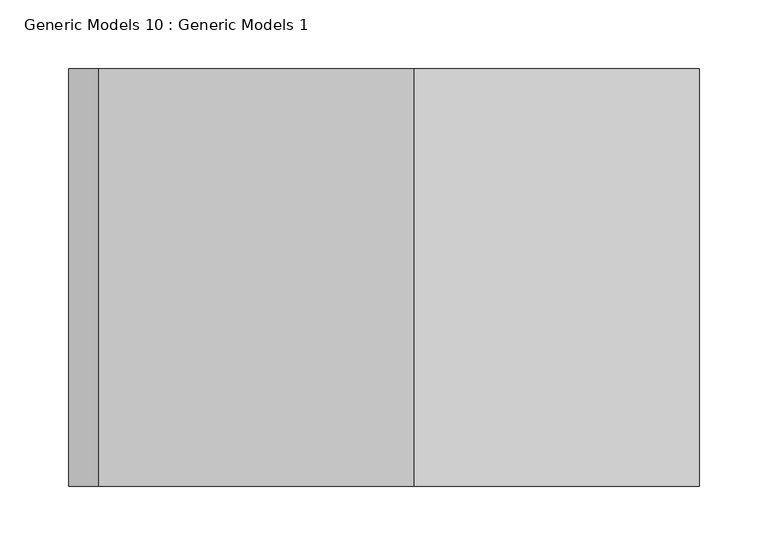
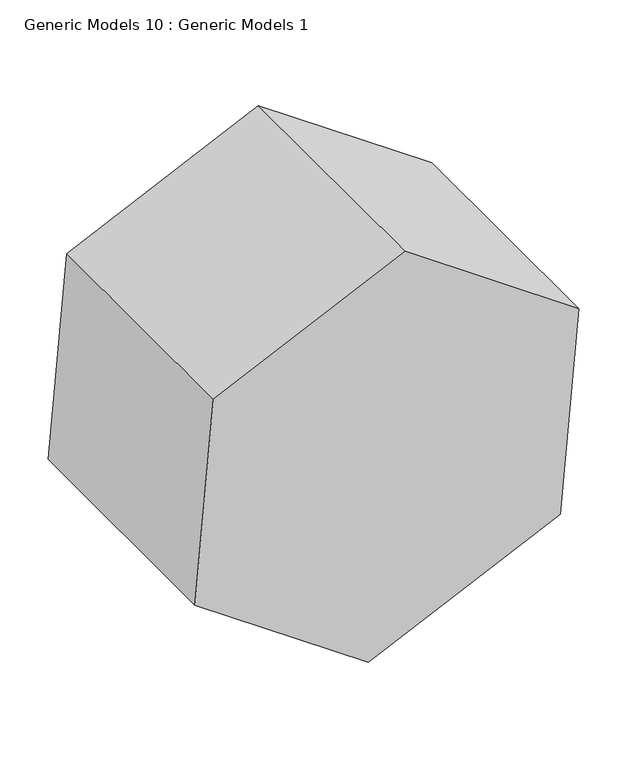
"""IFC4 building model written with IfcOpenShell, lengths in millimetres: proxy geometry, Generic Models 10 : Generic Models 1."""

from ifc_helpers import new_model, si_unit, frame, origin, place, context, project, spatial, polyline, outline, extrude, source, transform, mapped, element, save


def generic_models_10_generic_models_1_a884c7fe(model_context):
    return source(origin(), model_context, "Body", "SweptSolid", [
        extrude(outline(polyline([(833.1013393, 2028.4920945), (978.7897542, 1820.4274753), (871.4447157, 1590.2252974), (618.4112624, 1568.0877387), (472.7228475, 1776.152358), (580.067886, 2006.3545359), (833.1013393, 2028.4920945)])), frame((0.0, -10720.3372434, 0.0), z_axis=(0.0, 1.0, 0.0), x_axis=(0.0, 0.0, 1.0)), (0.0, 0.0, 1.0), 304.8),
    ])


if __name__ == "__main__":
    model = new_model("IFC4")
    model_context = context("Model", 3, world=origin())
    ifc_project = project(units=[si_unit("LENGTHUNIT", "METRE", prefix="MILLI")], contexts=[model_context])
    site = spatial("IfcSite", under=ifc_project)
    building = spatial("IfcBuilding", under=site)
    placement = place(None, origin())
    generic_models_10_generic_models_1_shape = generic_models_10_generic_models_1_a884c7fe(model_context)
    element("IfcBuildingElementProxy", 1, Name="Generic Models 10 : Generic Models 1", ObjectType="Generic Models 10 : Generic Models 1", at=placement, inside=building, context=model_context, shape_type="MappedRepresentation", body=[
        mapped(generic_models_10_generic_models_1_shape, transform((0.0, 0.0, 0.0), x_axis=(1.0, 0.0, 0.0), y_axis=(0.0, 1.0, 0.0), z_axis=(0.0, 0.0, 1.0))),
    ])
    save(model, "model.ifc")

# Revit data of these elements
# Element 1 (IfcBuildingElementProxy, "Generic Models 10 : Generic Models 1")
#   Materials on its faces: "Carpet (1)"
# Materials
#   "Carpet (1)": class "Carpet", colour RGB 124 80 67, transparency 0, Description = "Interior finish", Cost = 0
